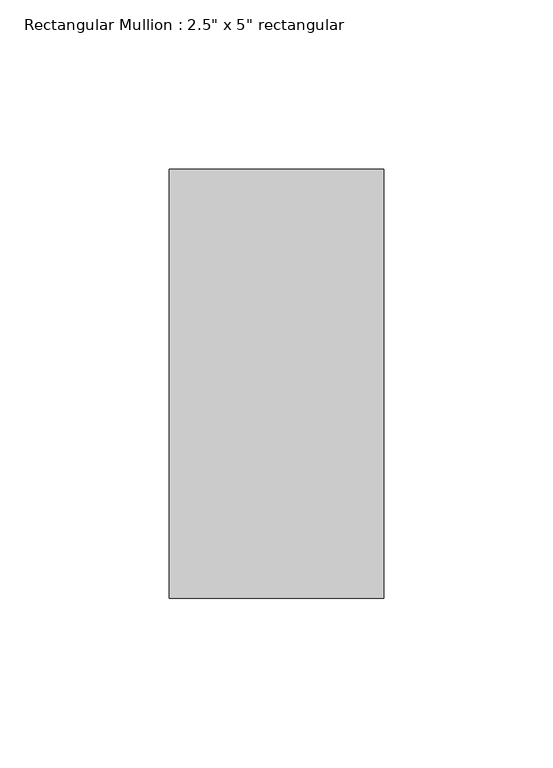
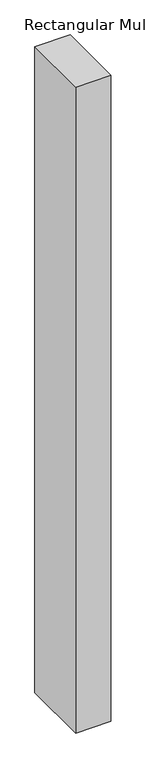
"""IFC4 building model written with IfcOpenShell, lengths in millimetres: member geometry."""

from ifc_helpers import new_model, si_unit, frame, origin, place, context, project, spatial, polyline, outline, extrude, source, transform, mapped, element, save


def member_3a6679d5(model_context):
    return source(origin(), model_context, "Body", "SweptSolid", [
        extrude(outline(polyline([(0.0, 63.5), (0.0, -63.5), (-63.5, -63.5), (-63.5, 63.5), (0.0, 63.5)])), frame((0.0, 0.0, -1230.8821304), z_axis=(0.0, 0.0, 1.0), x_axis=(1.0, 0.0, 0.0)), (0.0, 0.0, 1.0), 1230.8821304),
    ])


if __name__ == "__main__":
    model = new_model("IFC4")
    model_context = context("Model", 3, world=origin())
    ifc_project = project(units=[si_unit("LENGTHUNIT", "METRE", prefix="MILLI")], contexts=[model_context])
    site = spatial("IfcSite", under=ifc_project)
    building = spatial("IfcBuilding", under=site)
    placement = place(None, origin())
    member_shape = member_3a6679d5(model_context)
    element("IfcMember", 1, ObjectType="Rectangular Mullion : 2.5\" x 5\" rectangular", at=placement, inside=building, context=model_context, shape_type="MappedRepresentation", body=[
        mapped(member_shape, transform((0.0, 0.0, 0.0), x_axis=(1.0, 0.0, 0.0), y_axis=(0.0, 1.0, 0.0), z_axis=(0.0, 0.0, 1.0))),
    ])
    save(model, "model.ifc")

# Revit data of these elements
# Type "Rectangular Mullion : 2.5\" x 5\" rectangular"
#   built-in parameter 1007304 = 0.416667 (stored number, unit not read)
#   built-in parameter 1007301 = 0.104167 (stored number, unit not read)
#   built-in parameter 1007300 = 0.104167 (stored number, unit not read)
# Element 1 (IfcMember, "Rectangular Mullion : 2.5\" x 5\" rectangular")
#   Materials on its faces: "Aluminum"
# Materials
#   "Aluminum": class "Metal", colour RGB 247 247 247, transparency 0, Description = "Aluminum 6061", Cost = 0
